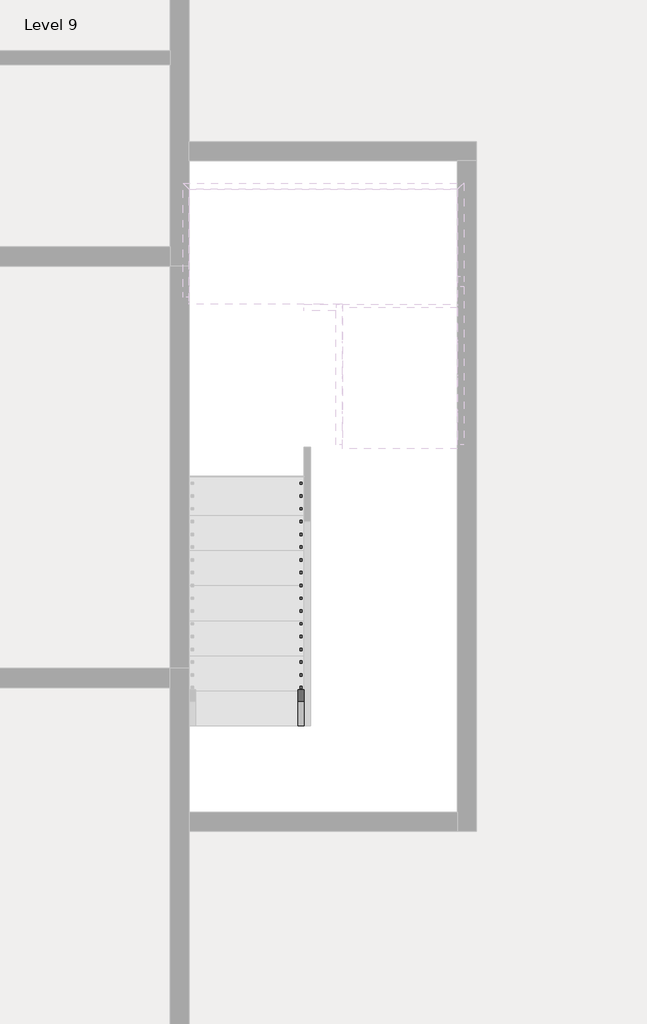
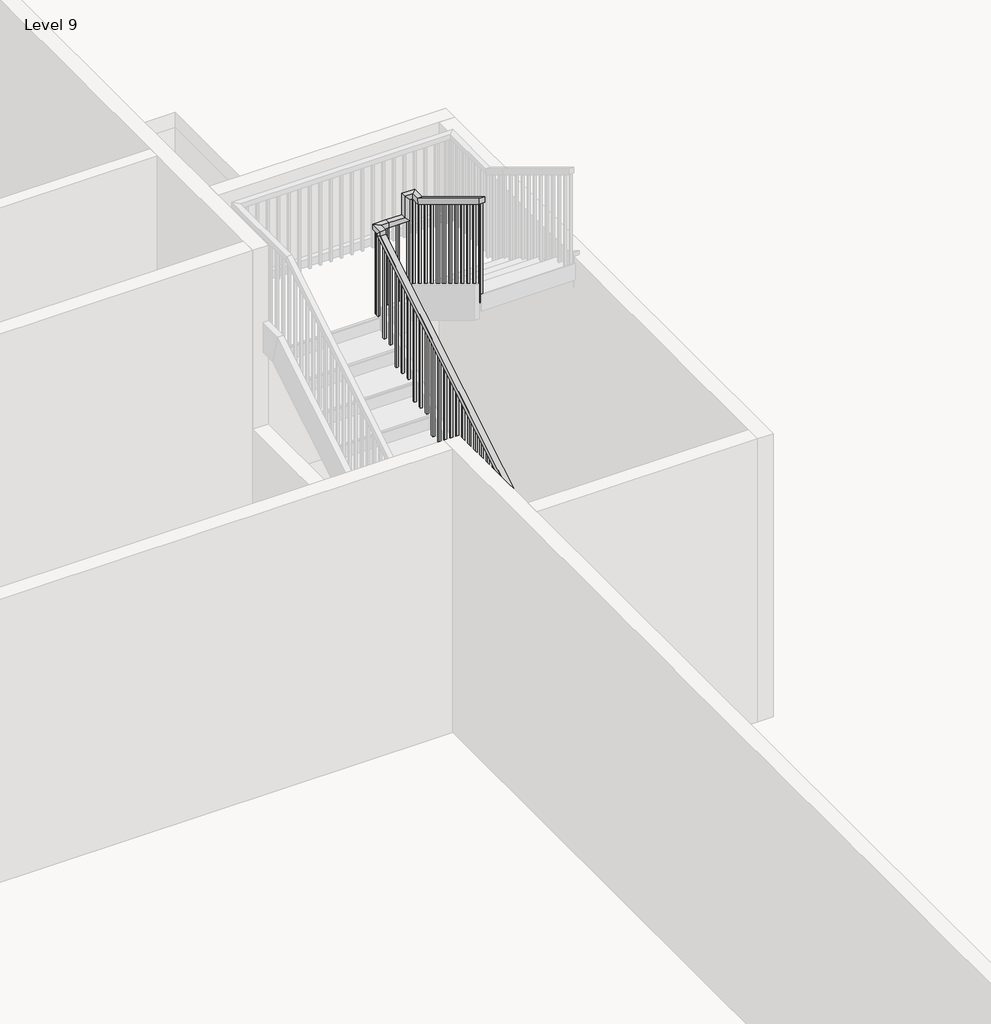
# One storey, part 7 of 8: 1 railing.
"""IFC4 building model written with IfcOpenShell, lengths in millimetres."""

from ifc_helpers import new_model, si_unit, frame, origin, place, context, project, spatial, polyline, outline, extrude, faceted_brep, element, save

model = new_model("IFC4")

# Units and contexts
model_context = context("Model", 3, world=origin())
ifc_project = project(units=[si_unit("LENGTHUNIT", "METRE", prefix="MILLI")], contexts=[model_context])

# Site, building, storey
site = spatial("IfcSite", under=ifc_project)
building = spatial("IfcBuilding", under=site)
storey = spatial("IfcBuildingStorey", under=building, Name="Level 9", Elevation=49618.6172466)

# Railing
placement = place(None, origin())
element("IfcRailing", 1, ObjectType="Handrail - Rectangular", at=placement, inside=storey, context=model_context, shape_type="SolidModel", body=[
    faceted_brep([(-2753.8415084, 19841.9216096, 50702.3505799), (-2753.8415084, 19841.9216096, 50642.9491197), (-2703.0415084, 19841.9216096, 50642.9491197), (-2703.0415084, 19841.9216096, 50702.3505799), (-2753.8415084, 23118.5216096, 52688.1687618), (-2753.8415084, 23169.3216096, 52659.5551803), (-2703.0415084, 23169.3216096, 52659.5551803), (-2703.0415084, 23118.5216096, 52688.1687618), (-2753.8415084, 23118.5216096, 52734.3505799), (-2753.8415084, 23169.3216096, 52683.5505799), (-2703.0415084, 23169.3216096, 52683.5505799), (-2703.0415084, 23118.5216096, 52734.3505799), (-2753.8415084, 23245.5216096, 52734.3505799), (-2753.8415084, 23245.5216096, 52683.5505799), (-2703.0415084, 23194.7216096, 52683.5505799), (-2703.0415084, 23194.7216096, 52734.3505799), (-2626.8415084, 23245.5216096, 52734.3505799), (-2626.8415084, 23245.5216096, 52683.5505799), (-2626.8415084, 23194.7216096, 52683.5505799), (-2626.8415084, 23194.7216096, 52734.3505799), (-2474.4415084, 23245.5216096, 52734.3505799), (-2423.6415084, 23245.5216096, 52683.5505799), (-2423.6415084, 23194.7216096, 52683.5505799), (-2474.4415084, 23194.7216096, 52734.3505799), (-2474.4415084, 23245.5216096, 52949.8657314), (-2423.6415084, 23245.5216096, 52899.0657314), (-2423.6415084, 23194.7216096, 52899.0657314), (-2474.4415084, 23194.7216096, 52949.8657314), (-2347.4415084, 23245.5216096, 52949.8657314), (-2347.4415084, 23245.5216096, 52899.0657314), (-2398.2415084, 23194.7216096, 52899.0657314), (-2398.2415084, 23194.7216096, 52949.8657314), (-2347.4415084, 23118.5216096, 52949.8657314), (-2347.4415084, 23104.3292002, 52899.0657314), (-2398.2415084, 23104.3292002, 52899.0657314), (-2398.2415084, 23118.5216096, 52949.8657314), (-2347.4415084, 22077.1216096, 53581.0172466), (-2398.2415084, 22077.1216096, 53581.0172466), (-2398.2415084, 22077.1216096, 53521.6157863), (-2347.4415084, 22077.1216096, 53521.6157863)], [[[0, 1, 2, 3]], [[1, 0, 4, 5]], [[2, 1, 5, 6]], [[3, 2, 6, 7]], [[0, 3, 7, 4]], [[5, 4, 8, 9]], [[6, 5, 9, 10]], [[7, 6, 10, 11]], [[4, 7, 11, 8]], [[9, 8, 12, 13]], [[10, 9, 13, 14]], [[11, 10, 14, 15]], [[8, 11, 15, 12]], [[13, 12, 16, 17]], [[14, 13, 17, 18]], [[15, 14, 18, 19]], [[12, 15, 19, 16]], [[17, 16, 20, 21]], [[18, 17, 21, 22]], [[19, 18, 22, 23]], [[16, 19, 23, 20]], [[21, 20, 24, 25]], [[22, 21, 25, 26]], [[23, 22, 26, 27]], [[20, 23, 27, 24]], [[25, 24, 28, 29]], [[26, 25, 29, 30]], [[27, 26, 30, 31]], [[24, 27, 31, 28]], [[29, 28, 32, 33]], [[30, 29, 33, 34]], [[31, 30, 34, 35]], [[28, 31, 35, 32]], [[36, 37, 38, 39]], [[33, 32, 36, 39]], [[34, 33, 39, 38]], [[35, 34, 38, 37]], [[32, 35, 37, 36]]]),
    extrude(outline(polyline([(22092.9966096, 53511.9945742), (22112.0466096, 53500.4491197), (22112.0466096, 52497.2839133), (22092.9966096, 52497.2839133), (22092.9966096, 53511.9945742)])), frame((-2382.3665084, 0.0, 0.0), z_axis=(1.0, 0.0, 0.0), x_axis=(0.0, 1.0, 0.0)), (0.0, 0.0, 1.0), 19.05),
    extrude(outline(polyline([(22194.5966096, 53450.4188166), (22213.6466096, 53438.8733621), (22213.6466096, 52497.2839133), (22194.5966096, 52497.2839133), (22194.5966096, 53450.4188166)])), frame((-2382.3665084, 0.0, 0.0), z_axis=(1.0, 0.0, 0.0), x_axis=(0.0, 1.0, 0.0)), (0.0, 0.0, 1.0), 19.05),
    extrude(outline(polyline([(22296.1966096, 53388.8430591), (22315.2466096, 53377.2976045), (22315.2466096, 52497.2839133), (22296.1966096, 52497.2839133), (22296.1966096, 53388.8430591)])), frame((-2382.3665084, 0.0, 0.0), z_axis=(1.0, 0.0, 0.0), x_axis=(0.0, 1.0, 0.0)), (0.0, 0.0, 1.0), 19.05),
    extrude(outline(polyline([(22397.7966096, 53327.2673015), (22416.8466096, 53315.721847), (22416.8466096, 52327.9505799), (22397.7966096, 52327.9505799), (22397.7966096, 53327.2673015)])), frame((-2382.3665084, 0.0, 0.0), z_axis=(1.0, 0.0, 0.0), x_axis=(0.0, 1.0, 0.0)), (0.0, 0.0, 1.0), 19.05),
    extrude(outline(polyline([(22499.3966096, 53265.6915439), (22518.4466096, 53254.1460894), (22518.4466096, 52327.9505799), (22499.3966096, 52327.9505799), (22499.3966096, 53265.6915439)])), frame((-2382.3665084, 0.0, 0.0), z_axis=(1.0, 0.0, 0.0), x_axis=(0.0, 1.0, 0.0)), (0.0, 0.0, 1.0), 19.05),
    extrude(outline(polyline([(22600.9966096, 53204.1157863), (22620.0466096, 53192.5703318), (22620.0466096, 52327.9505799), (22600.9966096, 52327.9505799), (22600.9966096, 53204.1157863)])), frame((-2382.3665084, 0.0, 0.0), z_axis=(1.0, 0.0, 0.0), x_axis=(0.0, 1.0, 0.0)), (0.0, 0.0, 1.0), 19.05),
    extrude(outline(polyline([(22702.5966096, 53142.5400288), (22721.6466096, 53130.9945742), (22721.6466096, 52158.6172466), (22702.5966096, 52158.6172466), (22702.5966096, 53142.5400288)])), frame((-2382.3665084, 0.0, 0.0), z_axis=(1.0, 0.0, 0.0), x_axis=(0.0, 1.0, 0.0)), (0.0, 0.0, 1.0), 19.05),
    extrude(outline(polyline([(22804.1966096, 53080.9642712), (22823.2466096, 53069.4188166), (22823.2466096, 52158.6172466), (22804.1966096, 52158.6172466), (22804.1966096, 53080.9642712)])), frame((-2382.3665084, 0.0, 0.0), z_axis=(1.0, 0.0, 0.0), x_axis=(0.0, 1.0, 0.0)), (0.0, 0.0, 1.0), 19.05),
    extrude(outline(polyline([(22905.7966096, 53019.3885136), (22924.8466096, 53007.8430591), (22924.8466096, 52158.6172466), (22905.7966096, 52158.6172466), (22905.7966096, 53019.3885136)])), frame((-2382.3665084, 0.0, 0.0), z_axis=(1.0, 0.0, 0.0), x_axis=(0.0, 1.0, 0.0)), (0.0, 0.0, 1.0), 19.05),
    extrude(outline(polyline([(23007.3966096, 52957.812756), (23026.4466096, 52946.2673015), (23026.4466096, 51989.2839133), (23007.3966096, 51989.2839133), (23007.3966096, 52957.812756)])), frame((-2382.3665084, 0.0, 0.0), z_axis=(1.0, 0.0, 0.0), x_axis=(0.0, 1.0, 0.0)), (0.0, 0.0, 1.0), 19.05),
    extrude(outline(polyline([(23108.9966096, 52896.2369985), (23128.0466096, 52884.6915439), (23128.0466096, 51989.2839133), (23108.9966096, 51989.2839133), (23108.9966096, 52896.2369985)])), frame((-2382.3665084, 0.0, 0.0), z_axis=(1.0, 0.0, 0.0), x_axis=(0.0, 1.0, 0.0)), (0.0, 0.0, 1.0), 19.05),
    extrude(outline(polyline([(-2433.1665084, 23210.5966096), (-2433.1665084, 23229.6466096), (-2414.1165084, 23229.6466096), (-2414.1165084, 23210.5966096), (-2433.1665084, 23210.5966096)])), frame((0.0, 0.0, 51819.9505799), z_axis=(0.0, 0.0, 1.0), x_axis=(1.0, 0.0, 0.0)), (0.0, 0.0, 1.0), 1079.1151515),
    extrude(outline(polyline([(-2534.7665084, 23210.5966096), (-2534.7665084, 23229.6466096), (-2515.7165084, 23229.6466096), (-2515.7165084, 23210.5966096), (-2534.7665084, 23210.5966096)])), frame((0.0, 0.0, 51819.9505799), z_axis=(0.0, 0.0, 1.0), x_axis=(1.0, 0.0, 0.0)), (0.0, 0.0, 1.0), 863.6),
    extrude(outline(polyline([(-2636.3665084, 23210.5966096), (-2636.3665084, 23229.6466096), (-2617.3165084, 23229.6466096), (-2617.3165084, 23210.5966096), (-2636.3665084, 23210.5966096)])), frame((0.0, 0.0, 51819.9505799), z_axis=(0.0, 0.0, 1.0), x_axis=(1.0, 0.0, 0.0)), (0.0, 0.0, 1.0), 863.6),
    extrude(outline(polyline([(-2718.9165084, 23185.1966096), (-2737.9665084, 23185.1966096), (-2737.9665084, 23204.2466096), (-2718.9165084, 23204.2466096), (-2718.9165084, 23185.1966096)])), frame((0.0, 0.0, 51819.9505799), z_axis=(0.0, 0.0, 1.0), x_axis=(1.0, 0.0, 0.0)), (0.0, 0.0, 1.0), 863.6),
    extrude(outline(polyline([(23083.5966096, 52607.6006348), (23102.6466096, 52619.1460894), (23102.6466096, 51650.6172466), (23083.5966096, 51650.6172466), (23083.5966096, 52607.6006348)])), frame((-2737.9665084, 0.0, 0.0), z_axis=(1.0, 0.0, 0.0), x_axis=(0.0, 1.0, 0.0)), (0.0, 0.0, 1.0), 19.05),
    extrude(outline(polyline([(22981.9966096, 52546.0248773), (23001.0466096, 52557.5703318), (23001.0466096, 51650.6172466), (22981.9966096, 51650.6172466), (22981.9966096, 52546.0248773)])), frame((-2737.9665084, 0.0, 0.0), z_axis=(1.0, 0.0, 0.0), x_axis=(0.0, 1.0, 0.0)), (0.0, 0.0, 1.0), 19.05),
    extrude(outline(polyline([(22880.3966096, 52484.4491197), (22899.4466096, 52495.9945742), (22899.4466096, 51481.2839133), (22880.3966096, 51481.2839133), (22880.3966096, 52484.4491197)])), frame((-2737.9665084, 0.0, 0.0), z_axis=(1.0, 0.0, 0.0), x_axis=(0.0, 1.0, 0.0)), (0.0, 0.0, 1.0), 19.05),
    extrude(outline(polyline([(22778.7966096, 52422.8733621), (22797.8466096, 52434.4188166), (22797.8466096, 51481.2839133), (22778.7966096, 51481.2839133), (22778.7966096, 52422.8733621)])), frame((-2737.9665084, 0.0, 0.0), z_axis=(1.0, 0.0, 0.0), x_axis=(0.0, 1.0, 0.0)), (0.0, 0.0, 1.0), 19.05),
    extrude(outline(polyline([(22677.1966096, 52361.2976045), (22696.2466096, 52372.8430591), (22696.2466096, 51481.2839133), (22677.1966096, 51481.2839133), (22677.1966096, 52361.2976045)])), frame((-2737.9665084, 0.0, 0.0), z_axis=(1.0, 0.0, 0.0), x_axis=(0.0, 1.0, 0.0)), (0.0, 0.0, 1.0), 19.05),
    extrude(outline(polyline([(22575.5966096, 52299.721847), (22594.6466096, 52311.2673015), (22594.6466096, 51311.9505799), (22575.5966096, 51311.9505799), (22575.5966096, 52299.721847)])), frame((-2737.9665084, 0.0, 0.0), z_axis=(1.0, 0.0, 0.0), x_axis=(0.0, 1.0, 0.0)), (0.0, 0.0, 1.0), 19.05),
    extrude(outline(polyline([(22473.9966096, 52238.1460894), (22493.0466096, 52249.6915439), (22493.0466096, 51311.9505799), (22473.9966096, 51311.9505799), (22473.9966096, 52238.1460894)])), frame((-2737.9665084, 0.0, 0.0), z_axis=(1.0, 0.0, 0.0), x_axis=(0.0, 1.0, 0.0)), (0.0, 0.0, 1.0), 19.05),
    extrude(outline(polyline([(22372.3966096, 52176.5703318), (22391.4466096, 52188.1157863), (22391.4466096, 51311.9505799), (22372.3966096, 51311.9505799), (22372.3966096, 52176.5703318)])), frame((-2737.9665084, 0.0, 0.0), z_axis=(1.0, 0.0, 0.0), x_axis=(0.0, 1.0, 0.0)), (0.0, 0.0, 1.0), 19.05),
    extrude(outline(polyline([(22270.7966096, 52114.9945742), (22289.8466096, 52126.5400288), (22289.8466096, 51142.6172466), (22270.7966096, 51142.6172466), (22270.7966096, 52114.9945742)])), frame((-2737.9665084, 0.0, 0.0), z_axis=(1.0, 0.0, 0.0), x_axis=(0.0, 1.0, 0.0)), (0.0, 0.0, 1.0), 19.05),
    extrude(outline(polyline([(22169.1966096, 52053.4188166), (22188.2466096, 52064.9642712), (22188.2466096, 51142.6172466), (22169.1966096, 51142.6172466), (22169.1966096, 52053.4188166)])), frame((-2737.9665084, 0.0, 0.0), z_axis=(1.0, 0.0, 0.0), x_axis=(0.0, 1.0, 0.0)), (0.0, 0.0, 1.0), 19.05),
    extrude(outline(polyline([(22067.5966096, 51991.8430591), (22086.6466096, 52003.3885136), (22086.6466096, 51142.6172466), (22067.5966096, 51142.6172466), (22067.5966096, 51991.8430591)])), frame((-2737.9665084, 0.0, 0.0), z_axis=(1.0, 0.0, 0.0), x_axis=(0.0, 1.0, 0.0)), (0.0, 0.0, 1.0), 19.05),
    extrude(outline(polyline([(21965.9966096, 51930.2673015), (21985.0466096, 51941.812756), (21985.0466096, 50973.2839133), (21965.9966096, 50973.2839133), (21965.9966096, 51930.2673015)])), frame((-2737.9665084, 0.0, 0.0), z_axis=(1.0, 0.0, 0.0), x_axis=(0.0, 1.0, 0.0)), (0.0, 0.0, 1.0), 19.05),
    extrude(outline(polyline([(21864.3966096, 51868.6915439), (21883.4466096, 51880.2369985), (21883.4466096, 50973.2839133), (21864.3966096, 50973.2839133), (21864.3966096, 51868.6915439)])), frame((-2737.9665084, 0.0, 0.0), z_axis=(1.0, 0.0, 0.0), x_axis=(0.0, 1.0, 0.0)), (0.0, 0.0, 1.0), 19.05),
    extrude(outline(polyline([(21762.7966096, 51807.1157863), (21781.8466096, 51818.6612409), (21781.8466096, 50803.9505799), (21762.7966096, 50803.9505799), (21762.7966096, 51807.1157863)])), frame((-2737.9665084, 0.0, 0.0), z_axis=(1.0, 0.0, 0.0), x_axis=(0.0, 1.0, 0.0)), (0.0, 0.0, 1.0), 19.05),
    extrude(outline(polyline([(21661.1966096, 51745.5400288), (21680.2466096, 51757.0854833), (21680.2466096, 50803.9505799), (21661.1966096, 50803.9505799), (21661.1966096, 51745.5400288)])), frame((-2737.9665084, 0.0, 0.0), z_axis=(1.0, 0.0, 0.0), x_axis=(0.0, 1.0, 0.0)), (0.0, 0.0, 1.0), 19.05),
    extrude(outline(polyline([(21559.5966096, 51683.9642712), (21578.6466096, 51695.5097257), (21578.6466096, 50803.9505799), (21559.5966096, 50803.9505799), (21559.5966096, 51683.9642712)])), frame((-2737.9665084, 0.0, 0.0), z_axis=(1.0, 0.0, 0.0), x_axis=(0.0, 1.0, 0.0)), (0.0, 0.0, 1.0), 19.05),
    extrude(outline(polyline([(21457.9966096, 51622.3885136), (21477.0466096, 51633.9339682), (21477.0466096, 50634.6172466), (21457.9966096, 50634.6172466), (21457.9966096, 51622.3885136)])), frame((-2737.9665084, 0.0, 0.0), z_axis=(1.0, 0.0, 0.0), x_axis=(0.0, 1.0, 0.0)), (0.0, 0.0, 1.0), 19.05),
    extrude(outline(polyline([(21356.3966096, 51560.812756), (21375.4466096, 51572.3582106), (21375.4466096, 50634.6172466), (21356.3966096, 50634.6172466), (21356.3966096, 51560.812756)])), frame((-2737.9665084, 0.0, 0.0), z_axis=(1.0, 0.0, 0.0), x_axis=(0.0, 1.0, 0.0)), (0.0, 0.0, 1.0), 19.05),
    extrude(outline(polyline([(21254.7966096, 51499.2369985), (21273.8466096, 51510.782453), (21273.8466096, 50634.6172466), (21254.7966096, 50634.6172466), (21254.7966096, 51499.2369985)])), frame((-2737.9665084, 0.0, 0.0), z_axis=(1.0, 0.0, 0.0), x_axis=(0.0, 1.0, 0.0)), (0.0, 0.0, 1.0), 19.05),
    extrude(outline(polyline([(21153.1966096, 51437.6612409), (21172.2466096, 51449.2066954), (21172.2466096, 50465.2839133), (21153.1966096, 50465.2839133), (21153.1966096, 51437.6612409)])), frame((-2737.9665084, 0.0, 0.0), z_axis=(1.0, 0.0, 0.0), x_axis=(0.0, 1.0, 0.0)), (0.0, 0.0, 1.0), 19.05),
    extrude(outline(polyline([(21051.5966096, 51376.0854833), (21070.6466096, 51387.6309379), (21070.6466096, 50465.2839133), (21051.5966096, 50465.2839133), (21051.5966096, 51376.0854833)])), frame((-2737.9665084, 0.0, 0.0), z_axis=(1.0, 0.0, 0.0), x_axis=(0.0, 1.0, 0.0)), (0.0, 0.0, 1.0), 19.05),
    extrude(outline(polyline([(20949.9966096, 51314.5097257), (20969.0466096, 51326.0551803), (20969.0466096, 50465.2839133), (20949.9966096, 50465.2839133), (20949.9966096, 51314.5097257)])), frame((-2737.9665084, 0.0, 0.0), z_axis=(1.0, 0.0, 0.0), x_axis=(0.0, 1.0, 0.0)), (0.0, 0.0, 1.0), 19.05),
    extrude(outline(polyline([(20848.3966096, 51252.9339682), (20867.4466096, 51264.4794227), (20867.4466096, 50295.9505799), (20848.3966096, 50295.9505799), (20848.3966096, 51252.9339682)])), frame((-2737.9665084, 0.0, 0.0), z_axis=(1.0, 0.0, 0.0), x_axis=(0.0, 1.0, 0.0)), (0.0, 0.0, 1.0), 19.05),
    extrude(outline(polyline([(20746.7966096, 51191.3582106), (20765.8466096, 51202.9036651), (20765.8466096, 50295.9505799), (20746.7966096, 50295.9505799), (20746.7966096, 51191.3582106)])), frame((-2737.9665084, 0.0, 0.0), z_axis=(1.0, 0.0, 0.0), x_axis=(0.0, 1.0, 0.0)), (0.0, 0.0, 1.0), 19.05),
    extrude(outline(polyline([(20645.1966096, 51129.782453), (20664.2466096, 51141.3279076), (20664.2466096, 50126.6172466), (20645.1966096, 50126.6172466), (20645.1966096, 51129.782453)])), frame((-2737.9665084, 0.0, 0.0), z_axis=(1.0, 0.0, 0.0), x_axis=(0.0, 1.0, 0.0)), (0.0, 0.0, 1.0), 19.05),
    extrude(outline(polyline([(20543.5966096, 51068.2066954), (20562.6466096, 51079.75215), (20562.6466096, 50126.6172466), (20543.5966096, 50126.6172466), (20543.5966096, 51068.2066954)])), frame((-2737.9665084, 0.0, 0.0), z_axis=(1.0, 0.0, 0.0), x_axis=(0.0, 1.0, 0.0)), (0.0, 0.0, 1.0), 19.05),
    extrude(outline(polyline([(20441.9966096, 51006.6309379), (20461.0466096, 51018.1763924), (20461.0466096, 50126.6172466), (20441.9966096, 50126.6172466), (20441.9966096, 51006.6309379)])), frame((-2737.9665084, 0.0, 0.0), z_axis=(1.0, 0.0, 0.0), x_axis=(0.0, 1.0, 0.0)), (0.0, 0.0, 1.0), 19.05),
    extrude(outline(polyline([(20340.3966096, 50945.0551803), (20359.4466096, 50956.6006348), (20359.4466096, 49957.2839133), (20340.3966096, 49957.2839133), (20340.3966096, 50945.0551803)])), frame((-2737.9665084, 0.0, 0.0), z_axis=(1.0, 0.0, 0.0), x_axis=(0.0, 1.0, 0.0)), (0.0, 0.0, 1.0), 19.05),
    extrude(outline(polyline([(20238.7966096, 50883.4794227), (20257.8466096, 50895.0248773), (20257.8466096, 49957.2839133), (20238.7966096, 49957.2839133), (20238.7966096, 50883.4794227)])), frame((-2737.9665084, 0.0, 0.0), z_axis=(1.0, 0.0, 0.0), x_axis=(0.0, 1.0, 0.0)), (0.0, 0.0, 1.0), 19.05),
    extrude(outline(polyline([(20137.1966096, 50821.9036651), (20156.2466096, 50833.4491197), (20156.2466096, 49957.2839133), (20137.1966096, 49957.2839133), (20137.1966096, 50821.9036651)])), frame((-2737.9665084, 0.0, 0.0), z_axis=(1.0, 0.0, 0.0), x_axis=(0.0, 1.0, 0.0)), (0.0, 0.0, 1.0), 19.05),
    extrude(outline(polyline([(20035.5966096, 50760.3279076), (20054.6466096, 50771.8733621), (20054.6466096, 49787.9505799), (20035.5966096, 49787.9505799), (20035.5966096, 50760.3279076)])), frame((-2737.9665084, 0.0, 0.0), z_axis=(1.0, 0.0, 0.0), x_axis=(0.0, 1.0, 0.0)), (0.0, 0.0, 1.0), 19.05),
    extrude(outline(polyline([(19933.9966096, 50698.75215), (19953.0466096, 50710.2976045), (19953.0466096, 49787.9505799), (19933.9966096, 49787.9505799), (19933.9966096, 50698.75215)])), frame((-2737.9665084, 0.0, 0.0), z_axis=(1.0, 0.0, 0.0), x_axis=(0.0, 1.0, 0.0)), (0.0, 0.0, 1.0), 19.05),
    extrude(outline(polyline([(-2382.3665084, 23210.5966096), (-2382.3665084, 23229.6466096), (-2363.3165084, 23229.6466096), (-2363.3165084, 23210.5966096), (-2382.3665084, 23210.5966096)])), frame((0.0, 0.0, 51819.9505799), z_axis=(0.0, 0.0, 1.0), x_axis=(1.0, 0.0, 0.0)), (0.0, 0.0, 1.0), 1079.1151515),
    extrude(outline(polyline([(-2718.9165084, 23210.5966096), (-2737.9665084, 23210.5966096), (-2737.9665084, 23229.6466096), (-2718.9165084, 23229.6466096), (-2718.9165084, 23210.5966096)])), frame((0.0, 0.0, 51819.9505799), z_axis=(0.0, 0.0, 1.0), x_axis=(1.0, 0.0, 0.0)), (0.0, 0.0, 1.0), 863.6),
    extrude(outline(polyline([(22077.1216096, 53521.6157863), (22096.1716096, 53510.0703318), (22096.1716096, 52497.2839133), (22077.1216096, 52497.2839133), (22077.1216096, 53521.6157863)])), frame((-2382.3665084, 0.0, 0.0), z_axis=(1.0, 0.0, 0.0), x_axis=(0.0, 1.0, 0.0)), (0.0, 0.0, 1.0), 19.05),
    extrude(outline(polyline([(19841.9216096, 50642.9491197), (19860.9716096, 50654.4945742), (19860.9716096, 49787.9505799), (19841.9216096, 49787.9505799), (19841.9216096, 50642.9491197)])), frame((-2737.9665084, 0.0, 0.0), z_axis=(1.0, 0.0, 0.0), x_axis=(0.0, 1.0, 0.0)), (0.0, 0.0, 1.0), 19.05),
])

save(model, "model.ifc")

# Revit data of these elements
# Type "Handrail - Rectangular"
#   Assembly Code = "C2010400"
#   built-in parameter 1008612 = 0.0416667 (stored number, unit not read)
#   built-in parameter 1008611 = 0.0416667 (stored number, unit not read)
#   built-in parameter 1008609 = 0.333333 (stored number, unit not read)
#   built-in parameter 1008604 = 0.166667 (stored number, unit not read)
#   built-in parameter 1008603 = 0.166667 (stored number, unit not read)
#   Railing Height = 3' - 0"
#   built-in parameter 1008630 = 2
#   built-in parameter 1008610 = 2
#   built-in parameter 1008618 = Baluster - Square : 3/4"
# Element 1 (IfcRailing, "Handrail - Rectangular")
#   Phase Created = New Construction
